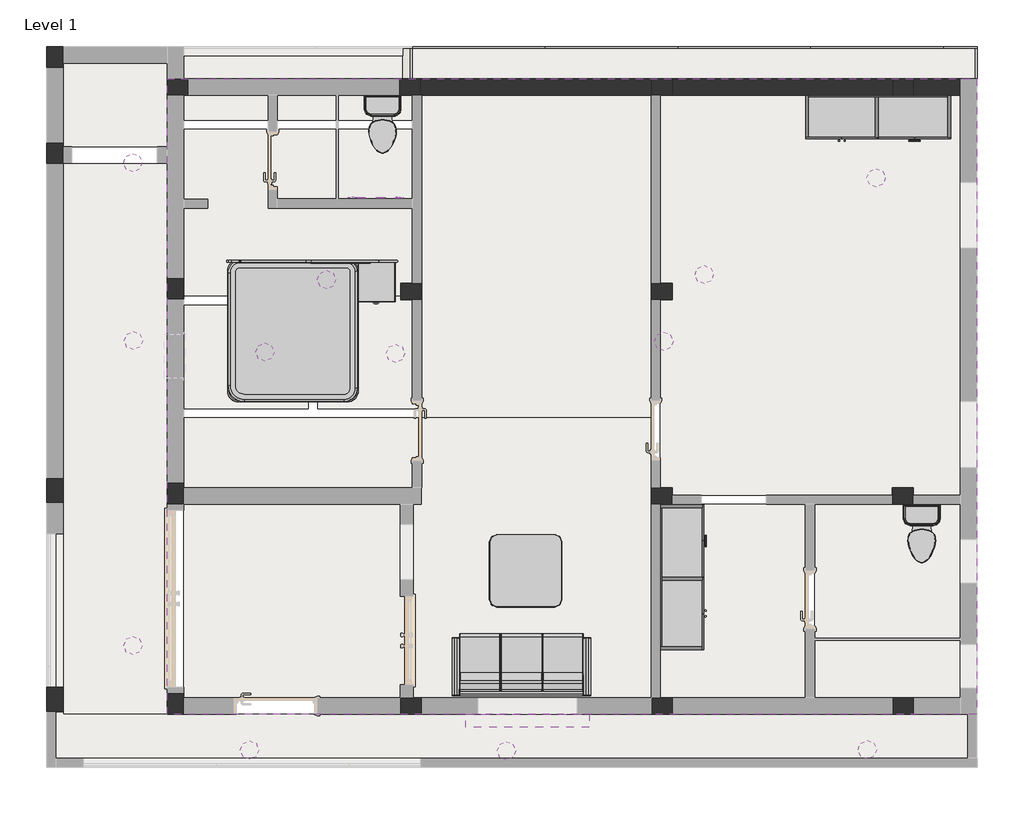
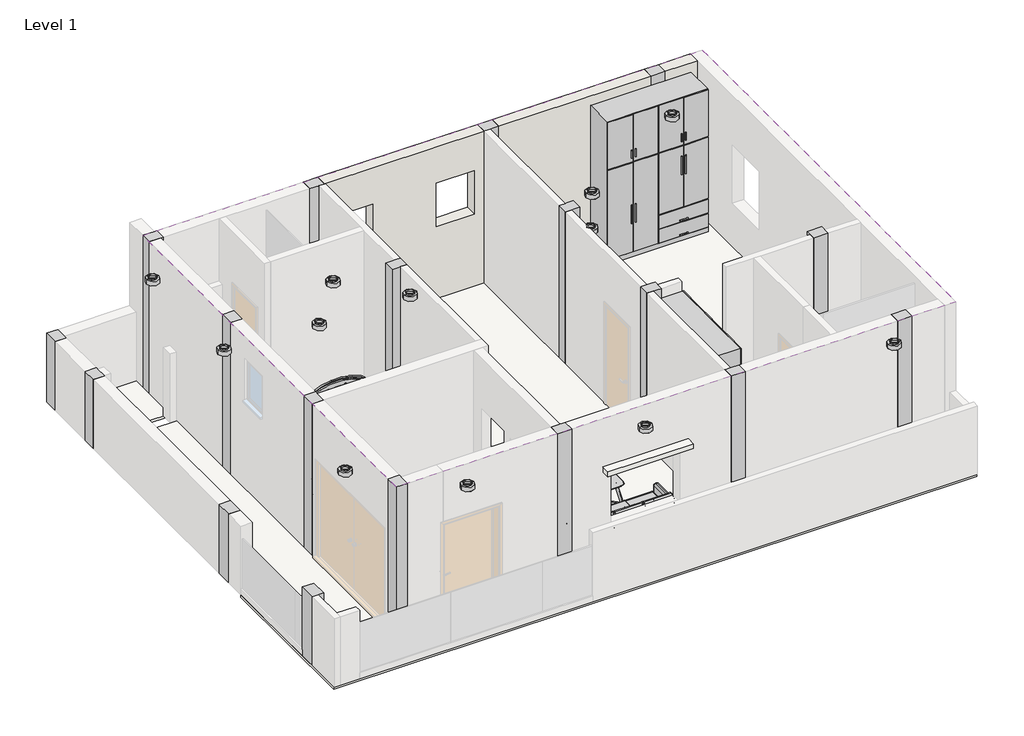
# One storey, part 2 of 2: 18 columns, 12 light fixtures, 7 plates, 6 slabs, 5 furniture elements, 4 walls, 3 flow terminals, 1 covering.
"""IFC4 building model written with IfcOpenShell, lengths in millimetres."""

from ifc_helpers import new_model, si_unit, frame, origin, place, context, project, spatial, polyline, outline, extrude, faceted_brep, transform, mapped, element, save
from components import concrete_rectangular_column_12_x_19_f479a93c, mirror_with_light_5960_af_41a2bd15, toilet_domestic_3d_toilet_domestic_3d_ba6479b0, toilet_domestic_3d_toilet_domestic_3d_30431060, furniture_2fc85b74, furniture_29a9adb8, furniture_57072a26, furniture_1wardrobe_6271_1wardrobe_6271_4dd35231, bed_design_8999_bed_design_8999_9c973422, bed_design_8999_bed_design_8999_e911dec7, coffee_table_16790_coffee_table_16790_723536ea, ceiling_light_flat_round_60w_120v_7c4c2a52, system_panel_glazed_6338a664, system_panel_glazed_bba74dcb, system_panel_glazed_77a7bb99, system_panel_glazed_06045eac

model = new_model("IFC4")

# Units and contexts
model_context = context("Model", 3, world=origin())
ifc_project = project(units=[si_unit("LENGTHUNIT", "METRE", prefix="MILLI")], contexts=[model_context])

# Site, building, storey
site = spatial("IfcSite", under=ifc_project)
building = spatial("IfcBuilding", under=site)
storey = spatial("IfcBuildingStorey", under=building, Name="Level 1", Elevation=3200.4)

# Columns
placement = place(None, origin())
element("IfcColumn", 1, ObjectType="Concrete-Rectangular-Column : 12 x 19", at=placement, inside=storey, context=model_context, shape_type="SweptSolid", body=[
    extrude(outline(polyline([(-12607.4604224, 5545.7949405), (-12607.4604224, 5253.6949405), (-12836.0604224, 5253.6949405), (-12836.0604224, 5545.7949405), (-12607.4604224, 5545.7949405)])), frame((0.0, 0.0, 3200.4), z_axis=(0.0, 0.0, 1.0), x_axis=(1.0, 0.0, 0.0)), (0.0, 0.0, 1.0), 1447.8),
])
element("IfcColumn", 2, ObjectType="Concrete-Rectangular-Column : 12 x 19", at=placement, inside=storey, context=model_context, shape_type="SweptSolid", body=[
    extrude(outline(polyline([(-12607.4604224, 4222.4988089), (-12607.4604224, 3930.3988089), (-12836.0604224, 3930.3988089), (-12836.0604224, 4222.4988089), (-12607.4604224, 4222.4988089)])), frame((0.0, 0.0, 3200.4), z_axis=(0.0, 0.0, 1.0), x_axis=(1.0, 0.0, 0.0)), (0.0, 0.0, 1.0), 1447.8),
])
element("IfcColumn", 3, ObjectType="Concrete-Rectangular-Column : 12 x 19", at=placement, inside=storey, context=model_context, shape_type="SweptSolid", body=[
    extrude(outline(polyline([(-10947.1858712, 2357.6455124), (-10947.1858712, 2065.5455124), (-11175.7858712, 2065.5455124), (-11175.7858712, 2357.6455124), (-10947.1858712, 2357.6455124)])), frame((0.0, 0.0, 3200.4), z_axis=(0.0, 0.0, 1.0), x_axis=(1.0, 0.0, 0.0)), (0.0, 0.0, 1.0), 3200.4),
])
element("IfcColumn", 4, ObjectType="Concrete-Rectangular-Column : 12 x 19", at=placement, inside=storey, context=model_context, shape_type="SweptSolid", body=[
    extrude(outline(polyline([(-10947.1858712, -467.0796054), (-10947.1858712, -759.1796054), (-11175.7858712, -759.1796054), (-11175.7858712, -467.0796054), (-10947.1858712, -467.0796054)])), frame((0.0, 0.0, 3200.4), z_axis=(0.0, 0.0, 1.0), x_axis=(1.0, 0.0, 0.0)), (0.0, 0.0, 1.0), 3200.4),
])
element("IfcColumn", 5, ObjectType="Concrete-Rectangular-Column : 12 x 19", at=placement, inside=storey, context=model_context, shape_type="Brep", body=[
    faceted_brep([(-10947.1858712, -3362.6796054, 3200.4), (-10947.1858712, -3426.1796054, 3200.4), (-10947.1858712, -3654.7796054, 3200.4), (-11175.7858712, -3654.7796054, 3200.4), (-11175.7858712, -3362.6796054, 3200.4), (-10947.1858712, -3362.6796054, 6400.8), (-10947.1858712, -3426.1796054, 6400.8), (-10947.1858712, -3654.7796054, 6400.8), (-11175.7858712, -3654.7796054, 6400.8), (-11175.7858712, -3362.6796054, 6400.8)], [[[0, 1, 2, 3, 4]], [[5, 6, 7, 2, 1, 0]], [[7, 8, 3, 2]], [[8, 9, 4, 3]], [[9, 5, 0, 4]], [[5, 9, 8, 7, 6]]]),
])
element("IfcColumn", 6, ObjectType="Concrete-Rectangular-Column : 12 x 19", at=placement, inside=storey, context=model_context, shape_type="SweptSolid", body=[
    extrude(outline(polyline([(-7668.2445565, -3654.7796054), (-7960.3445565, -3654.7796054), (-7960.3445565, -3426.1796054), (-7668.2445565, -3426.1796054), (-7668.2445565, -3654.7796054)])), frame((0.0, 0.0, 3200.4), z_axis=(0.0, 0.0, 1.0), x_axis=(1.0, 0.0, 0.0)), (0.0, 0.0, 1.0), 3200.4),
])
element("IfcColumn", 7, ObjectType="Concrete-Rectangular-Column : 12 x 19", at=placement, inside=storey, context=model_context, shape_type="SweptSolid", body=[
    extrude(outline(polyline([(-4204.83523, -3654.7796054), (-4496.93523, -3654.7796054), (-4496.93523, -3426.1796054), (-4204.83523, -3426.1796054), (-4204.83523, -3654.7796054)])), frame((0.0, 0.0, 3200.4), z_axis=(0.0, 0.0, 1.0), x_axis=(1.0, 0.0, 0.0)), (0.0, 0.0, 1.0), 3200.4),
])
element("IfcColumn", 8, ObjectType="Concrete-Rectangular-Column : 12 x 19", at=placement, inside=storey, context=model_context, shape_type="SweptSolid", body=[
    extrude(outline(polyline([(-883.78523, -3654.7796054), (-1175.88523, -3654.7796054), (-1175.88523, -3426.1796054), (-883.78523, -3426.1796054), (-883.78523, -3654.7796054)])), frame((0.0, 0.0, 3200.4), z_axis=(0.0, 0.0, 1.0), x_axis=(1.0, 0.0, 0.0)), (0.0, 0.0, 1.0), 3200.4),
])
element("IfcColumn", 9, ObjectType="Concrete-Rectangular-Column : 12 x 19", at=placement, inside=storey, context=model_context, shape_type="SweptSolid", body=[
    extrude(outline(polyline([(-890.13523, -764.1797525), (-1182.23523, -764.1797525), (-1182.23523, -535.5797525), (-890.13523, -535.5797525), (-890.13523, -764.1797525)])), frame((0.0, 0.0, 3200.4), z_axis=(0.0, 0.0, 1.0), x_axis=(1.0, 0.0, 0.0)), (0.0, 0.0, 1.0), 3200.4),
])
element("IfcColumn", 10, ObjectType="Concrete-Rectangular-Column : 12 x 19", at=placement, inside=storey, context=model_context, shape_type="SweptSolid", body=[
    extrude(outline(polyline([(-883.78523, 4873.0327475), (-1175.88523, 4873.0327475), (-1175.88523, 5101.6327475), (-883.78523, 5101.6327475), (-883.78523, 4873.0327475)])), frame((0.0, 0.0, 3200.4), z_axis=(0.0, 0.0, 1.0), x_axis=(1.0, 0.0, 0.0)), (0.0, 0.0, 1.0), 3200.4),
])
element("IfcColumn", 11, ObjectType="Concrete-Rectangular-Column : 12 x 19", at=placement, inside=storey, context=model_context, shape_type="SweptSolid", body=[
    extrude(outline(polyline([(-4207.375513, 4873.0327475), (-4499.475513, 4873.0327475), (-4499.475513, 5101.6327475), (-4207.375513, 5101.6327475), (-4207.375513, 4873.0327475)])), frame((0.0, 0.0, 3200.4), z_axis=(0.0, 0.0, 1.0), x_axis=(1.0, 0.0, 0.0)), (0.0, 0.0, 1.0), 3200.4),
])
element("IfcColumn", 12, ObjectType="Concrete-Rectangular-Column : 12 x 19", at=placement, inside=storey, context=model_context, shape_type="SweptSolid", body=[
    extrude(outline(polyline([(-7680.825513, 4873.0327475), (-7972.925513, 4873.0327475), (-7972.925513, 5101.6327475), (-7680.825513, 5101.6327475), (-7680.825513, 4873.0327475)])), frame((0.0, 0.0, 3200.4), z_axis=(0.0, 0.0, 1.0), x_axis=(1.0, 0.0, 0.0)), (0.0, 0.0, 1.0), 3200.4),
])
element("IfcColumn", 13, ObjectType="Concrete-Rectangular-Column : 12 x 19", at=placement, inside=storey, context=model_context, shape_type="SweptSolid", body=[
    extrude(outline(polyline([(-10883.6959332, 4876.8926487), (-11175.7959332, 4876.8926487), (-11175.7959332, 5105.4926487), (-10883.6959332, 5105.4926487), (-10883.6959332, 4876.8926487)])), frame((0.0, 0.0, 3200.4), z_axis=(0.0, 0.0, 1.0), x_axis=(1.0, 0.0, 0.0)), (0.0, 0.0, 1.0), 3200.4),
])
concrete_rectangular_column_12_x_19_shape = concrete_rectangular_column_12_x_19_f479a93c(model_context)
element("IfcColumn", 14, ObjectType="Concrete-Rectangular-Column : 12 x 19", at=placement, inside=storey, context=model_context, shape_type="MappedRepresentation", body=[
    mapped(concrete_rectangular_column_12_x_19_shape, transform((-7812.2134981, 2171.1077475, 0.0), x_axis=(0.0, -1.0, 0.0), y_axis=(1.0, 0.0, 0.0), z_axis=(0.0, 0.0, 1.0))),
])
element("IfcColumn", 15, ObjectType="Concrete-Rectangular-Column : 12 x 19", at=placement, inside=storey, context=model_context, shape_type="MappedRepresentation", body=[
    mapped(concrete_rectangular_column_12_x_19_shape, transform((-4360.0560272, 2171.1077475, 0.0), x_axis=(0.0, -1.0, 0.0), y_axis=(1.0, 0.0, 0.0), z_axis=(0.0, 0.0, 1.0))),
])
element("IfcColumn", 16, ObjectType="Concrete-Rectangular-Column : 12 x 19", at=placement, inside=storey, context=model_context, shape_type="MappedRepresentation", body=[
    mapped(concrete_rectangular_column_12_x_19_shape, transform((-4360.0560272, -649.8797525, 0.0), x_axis=(0.0, -1.0, 0.0), y_axis=(1.0, 0.0, 0.0), z_axis=(0.0, 0.0, 1.0))),
])
element("IfcColumn", 17, ObjectType="Concrete-Rectangular-Column : 12 x 20", at=placement, inside=storey, context=model_context, shape_type="SweptSolid", body=[
    extrude(outline(polyline([(-12607.4604224, -404.5396501), (-12607.4604224, -747.4396501), (-12836.0604224, -747.4396501), (-12836.0604224, -404.5396501), (-12607.4604224, -404.5396501)])), frame((0.0, 0.0, 3200.4), z_axis=(0.0, 0.0, 1.0), x_axis=(1.0, 0.0, 0.0)), (0.0, 0.0, 1.0), 1447.8),
])
element("IfcColumn", 18, ObjectType="Concrete-Rectangular-Column : 12 x 20", at=placement, inside=storey, context=model_context, shape_type="SweptSolid", body=[
    extrude(outline(polyline([(-12607.4604224, -3281.0896501), (-12607.4604224, -3623.9896501), (-12836.0604224, -3623.9896501), (-12836.0604224, -3281.0896501), (-12607.4604224, -3281.0896501)])), frame((0.0, 0.0, 3200.4), z_axis=(0.0, 0.0, 1.0), x_axis=(1.0, 0.0, 0.0)), (0.0, 0.0, 1.0), 1447.8),
])

# Covering
element("IfcCovering", 19, ObjectType="Plain", at=placement, inside=storey, context=model_context, shape_type="Brep", body=[
    faceted_brep([(-13.83523, 5101.6327475, 6477.0), (-11175.7858712, 5101.6327475, 6477.0), (-11175.7858712, -3654.7796054, 6477.0), (-242.43523, -3654.7796054, 6477.0), (-13.83523, -3654.7796054, 6477.0), (-13.83523, 5101.6327475, 6400.8), (-13.83523, -3654.7796054, 6400.8), (-11175.7858712, -3654.7796054, 6400.8), (-11175.7858712, 5101.6327475, 6400.8)], [[[0, 1, 2, 3, 4]], [[5, 6, 7, 8]], [[1, 0, 5, 8]], [[2, 1, 8, 7]], [[4, 3, 2, 7, 6]], [[0, 4, 6, 5]]]),
])

# Flow terminals
mirror_with_light_5960_af_shape = mirror_with_light_5960_af_41a2bd15(model_context)
element("IfcFlowTerminal", 20, ObjectType="Mirror_with_Light_5960 : AF", at=placement, inside=storey, context=model_context, shape_type="MappedRepresentation", body=[
    mapped(mirror_with_light_5960_af_shape, transform((-8322.2830614, 3383.1639975, 3505.2), x_axis=(1.0, 0.0, 0.0), y_axis=(0.0, 1.0, 0.0), z_axis=(0.0, 0.0, 1.0))),
])
toilet_domestic_3d_toilet_domestic_3d_shape = toilet_domestic_3d_toilet_domestic_3d_ba6479b0(model_context)
toilet_domestic_3d_toilet_domestic_3d_2_shape = toilet_domestic_3d_toilet_domestic_3d_30431060(model_context)
element("IfcFlowTerminal", 21, ObjectType="Toilet-Domestic-3D : Toilet-Domestic-3D", at=placement, inside=storey, context=model_context, shape_type="MappedRepresentation", body=[
    mapped(toilet_domestic_3d_toilet_domestic_3d_shape, transform((-775.83523, -1258.8757798, 3200.4), x_axis=(1.0, 0.0, 0.0), y_axis=(0.0, 1.0, 0.0), z_axis=(0.0, 0.0, 1.0))),
    mapped(toilet_domestic_3d_toilet_domestic_3d_2_shape, transform((-775.83523, -1258.8757798, 3200.4), x_axis=(1.0, 0.0, 0.0), y_axis=(0.0, 1.0, 0.0), z_axis=(0.0, 0.0, 1.0))),
])
element("IfcFlowTerminal", 22, ObjectType="Toilet-Domestic-3D : Toilet-Domestic-3D", at=placement, inside=storey, context=model_context, shape_type="MappedRepresentation", body=[
    mapped(toilet_domestic_3d_toilet_domestic_3d_shape, transform((-8205.9134981, 4382.1966213, 3200.4), x_axis=(1.0, 0.0, 0.0), y_axis=(0.0, 1.0, 0.0), z_axis=(0.0, 0.0, 1.0))),
    mapped(toilet_domestic_3d_toilet_domestic_3d_2_shape, transform((-8205.9134981, 4382.1966213, 3200.4), x_axis=(1.0, 0.0, 0.0), y_axis=(0.0, 1.0, 0.0), z_axis=(0.0, 0.0, 1.0))),
])

# Furniture
furniture_shape = furniture_2fc85b74(model_context)
furniture_2_shape = furniture_29a9adb8(model_context)
furniture_3_shape = furniture_57072a26(model_context)
element("IfcFurniture", 23, at=placement, inside=storey, context=model_context, shape_type="MappedRepresentation", body=[
    mapped(furniture_shape, transform((-6291.7541525, -2600.6796054, 3200.4), x_axis=(-1.0, 0.0, 0.0), y_axis=(0.0, -1.0, 0.0), z_axis=(0.0, 0.0, 1.0))),
    mapped(furniture_2_shape, transform((-6291.7541525, -2600.6796054, 3200.4), x_axis=(-1.0, 0.0, 0.0), y_axis=(0.0, -1.0, 0.0), z_axis=(0.0, 0.0, 1.0))),
    mapped(furniture_3_shape, transform((-6291.7541525, -2600.6796054, 3200.4), x_axis=(-1.0, 0.0, 0.0), y_axis=(0.0, -1.0, 0.0), z_axis=(0.0, 0.0, 1.0))),
])
furniture_1wardrobe_6271_1wardrobe_6271_shape = furniture_1wardrobe_6271_1wardrobe_6271_4dd35231(model_context)
element("IfcFurniture", 24, ObjectType="1Wardrobe_6271 : 1Wardrobe_6271", at=placement, inside=storey, context=model_context, shape_type="MappedRepresentation", body=[
    mapped(furniture_1wardrobe_6271_1wardrobe_6271_shape, transform((-2376.03523, 4873.0327475, 3200.4), x_axis=(1.0, 0.0, 0.0), y_axis=(0.0, 1.0, 0.0), z_axis=(0.0, 0.0, 1.0))),
])
element("IfcFurniture", 25, ObjectType="1Wardrobe_6271 : 1Wardrobe_6271", at=placement, inside=storey, context=model_context, shape_type="MappedRepresentation", body=[
    mapped(furniture_1wardrobe_6271_1wardrobe_6271_shape, transform((-4379.1060272, -2766.7129976, 3200.4), x_axis=(0.0, 1.0, 0.0), y_axis=(-1.0, 0.0, 0.0), z_axis=(0.0, 0.0, 1.0))),
])
bed_design_8999_bed_design_8999_shape = bed_design_8999_bed_design_8999_9c973422(model_context)
bed_design_8999_bed_design_8999_2_shape = bed_design_8999_bed_design_8999_e911dec7(model_context)
element("IfcFurniture", 26, ObjectType="BED_DESIGN_8999 : BED_DESIGN_8999", at=placement, inside=storey, context=model_context, shape_type="MappedRepresentation", body=[
    mapped(bed_design_8999_bed_design_8999_shape, transform((-9240.9634981, 652.6639975, 3200.4), x_axis=(1.0, 0.0, 0.0), y_axis=(0.0, 1.0, 0.0), z_axis=(0.0, 0.0, 1.0))),
    mapped(bed_design_8999_bed_design_8999_2_shape, transform((-9240.9634981, 652.6639975, 3200.4), x_axis=(1.0, 0.0, 0.0), y_axis=(0.0, 1.0, 0.0), z_axis=(0.0, 0.0, 1.0))),
])
coffee_table_16790_coffee_table_16790_shape = coffee_table_16790_coffee_table_16790_723536ea(model_context)
element("IfcFurniture", 27, ObjectType="Coffee_Table_16790 : Coffee_Table_16790", at=placement, inside=storey, context=model_context, shape_type="MappedRepresentation", body=[
    mapped(coffee_table_16790_coffee_table_16790_shape, transform((-6233.3060272, -1678.5797525, 3200.4), x_axis=(0.0, 1.0, 0.0), y_axis=(-1.0, 0.0, 0.0), z_axis=(0.0, 0.0, 1.0))),
])

# Light fixtures
ceiling_light_flat_round_60w_120v_shape = ceiling_light_flat_round_60w_120v_7c4c2a52(model_context)
element("IfcLightFixture", 28, ObjectType="Ceiling Light - Flat Round : 60W - 120V", at=placement, inside=storey, context=model_context, shape_type="MappedRepresentation", body=[
    mapped(ceiling_light_flat_round_60w_120v_shape, transform((-8976.6249266, 2333.1202007, 3962.4), x_axis=(1.0, 0.0, 0.0), y_axis=(0.0, 1.0, 0.0), z_axis=(0.0, 0.0, 1.0))),
])
element("IfcLightFixture", 29, ObjectType="Ceiling Light - Flat Round : 60W - 120V", at=placement, inside=storey, context=model_context, shape_type="MappedRepresentation", body=[
    mapped(ceiling_light_flat_round_60w_120v_shape, transform((-9826.6973698, 1336.4578052, 3962.4), x_axis=(1.0, 0.0, 0.0), y_axis=(0.0, 1.0, 0.0), z_axis=(0.0, 0.0, 1.0))),
])
element("IfcLightFixture", 30, ObjectType="Ceiling Light - Flat Round : 60W - 120V", at=placement, inside=storey, context=model_context, shape_type="MappedRepresentation", body=[
    mapped(ceiling_light_flat_round_60w_120v_shape, transform((-8027.2127557, 1317.1708554, 3962.4), x_axis=(1.0, 0.0, 0.0), y_axis=(0.0, 1.0, 0.0), z_axis=(0.0, 0.0, 1.0))),
])
element("IfcLightFixture", 31, ObjectType="Ceiling Light - Flat Round : 60W - 120V", at=placement, inside=storey, context=model_context, shape_type="MappedRepresentation", body=[
    mapped(ceiling_light_flat_round_60w_120v_shape, transform((-1403.7470603, 3737.3422943, 3962.4), x_axis=(1.0, 0.0, 0.0), y_axis=(0.0, 1.0, 0.0), z_axis=(0.0, 0.0, 1.0))),
])
element("IfcLightFixture", 32, ObjectType="Ceiling Light - Flat Round : 60W - 120V", at=placement, inside=storey, context=model_context, shape_type="MappedRepresentation", body=[
    mapped(ceiling_light_flat_round_60w_120v_shape, transform((-4329.6170331, 1484.2886755, 3962.4), x_axis=(1.0, 0.0, 0.0), y_axis=(0.0, 1.0, 0.0), z_axis=(0.0, 0.0, 1.0))),
])
element("IfcLightFixture", 33, ObjectType="Ceiling Light - Flat Round : 60W - 120V", at=placement, inside=storey, context=model_context, shape_type="MappedRepresentation", body=[
    mapped(ceiling_light_flat_round_60w_120v_shape, transform((-3772.5595971, 2403.8335381, 3962.4), x_axis=(1.0, 0.0, 0.0), y_axis=(0.0, 1.0, 0.0), z_axis=(0.0, 0.0, 1.0))),
])
element("IfcLightFixture", 34, ObjectType="Ceiling Light - Flat Round : 60W - 277V", at=placement, inside=storey, context=model_context, shape_type="MappedRepresentation", body=[
    mapped(ceiling_light_flat_round_60w_120v_shape, transform((-11647.8170744, 3944.8565115, 3962.4), x_axis=(1.0, 0.0, 0.0), y_axis=(0.0, 1.0, 0.0), z_axis=(0.0, 0.0, 1.0))),
])
element("IfcLightFixture", 35, ObjectType="Ceiling Light - Flat Round : 60W - 277V", at=placement, inside=storey, context=model_context, shape_type="MappedRepresentation", body=[
    mapped(ceiling_light_flat_round_60w_120v_shape, transform((-11638.1699852, 1493.9262651, 3962.4), x_axis=(1.0, 0.0, 0.0), y_axis=(0.0, 1.0, 0.0), z_axis=(0.0, 0.0, 1.0))),
])
element("IfcLightFixture", 36, ObjectType="Ceiling Light - Flat Round : 60W - 277V", at=placement, inside=storey, context=model_context, shape_type="MappedRepresentation", body=[
    mapped(ceiling_light_flat_round_60w_120v_shape, transform((-11644.9561662, -2707.9806169, 3962.4), x_axis=(1.0, 0.0, 0.0), y_axis=(0.0, 1.0, 0.0), z_axis=(0.0, 0.0, 1.0))),
])
element("IfcLightFixture", 37, ObjectType="Ceiling Light - Flat Round : 60W - 277V", at=placement, inside=storey, context=model_context, shape_type="MappedRepresentation", body=[
    mapped(ceiling_light_flat_round_60w_120v_shape, transform((-10037.5878836, -4148.1202674, 3962.4), x_axis=(1.0, 0.0, 0.0), y_axis=(0.0, 1.0, 0.0), z_axis=(0.0, 0.0, 1.0))),
])
element("IfcLightFixture", 38, ObjectType="Ceiling Light - Flat Round : 60W - 277V", at=placement, inside=storey, context=model_context, shape_type="MappedRepresentation", body=[
    mapped(ceiling_light_flat_round_60w_120v_shape, transform((-6498.1676871, -4159.8217019, 3962.4), x_axis=(1.0, 0.0, 0.0), y_axis=(0.0, 1.0, 0.0), z_axis=(0.0, 0.0, 1.0))),
])
element("IfcLightFixture", 39, ObjectType="Ceiling Light - Flat Round : 60W - 277V", at=placement, inside=storey, context=model_context, shape_type="MappedRepresentation", body=[
    mapped(ceiling_light_flat_round_60w_120v_shape, transform((-1525.3967065, -4143.4135843, 3962.4), x_axis=(1.0, 0.0, 0.0), y_axis=(0.0, 1.0, 0.0), z_axis=(0.0, 0.0, 1.0))),
])

# Plates
system_panel_glazed_shape = system_panel_glazed_6338a664(model_context)
element("IfcPlate", 40, ObjectType="System Panel : Glazed", at=placement, inside=storey, context=model_context, shape_type="MappedRepresentation", body=[
    mapped(system_panel_glazed_shape, transform((-6883.885871, 5497.0125322, 3200.4), x_axis=(1.0, 0.0, 0.0), y_axis=(0.0, 1.0, 0.0), z_axis=(0.0, 0.0, 1.0))),
])
element("IfcPlate", 41, ObjectType="System Panel : Glazed", at=placement, inside=storey, context=model_context, shape_type="MappedRepresentation", body=[
    mapped(system_panel_glazed_shape, transform((-5053.8858709, 5497.0125322, 3200.4), x_axis=(1.0, 0.0, 0.0), y_axis=(0.0, 1.0, 0.0), z_axis=(0.0, 0.0, 1.0))),
])
element("IfcPlate", 42, ObjectType="System Panel : Glazed", at=placement, inside=storey, context=model_context, shape_type="MappedRepresentation", body=[
    mapped(system_panel_glazed_shape, transform((-3223.8858709, 5497.0125322, 3200.4), x_axis=(1.0, 0.0, 0.0), y_axis=(0.0, 1.0, 0.0), z_axis=(0.0, 0.0, 1.0))),
])
element("IfcPlate", 43, ObjectType="System Panel : Glazed", at=placement, inside=storey, context=model_context, shape_type="MappedRepresentation", body=[
    mapped(system_panel_glazed_shape, transform((-1393.8858709, 5497.0125322, 3200.4), x_axis=(1.0, 0.0, 0.0), y_axis=(0.0, 1.0, 0.0), z_axis=(0.0, 0.0, 1.0))),
])
system_panel_glazed_2_shape = system_panel_glazed_bba74dcb(model_context)
element("IfcPlate", 44, ObjectType="System Panel : Glazed", at=placement, inside=storey, context=model_context, shape_type="MappedRepresentation", body=[
    mapped(system_panel_glazed_2_shape, transform((-7848.3858712, 5311.357594, 3200.4), x_axis=(0.0, -1.0, 0.0), y_axis=(1.0, 0.0, 0.0), z_axis=(0.0, 0.0, 1.0))),
])
system_panel_glazed_3_shape = system_panel_glazed_77a7bb99(model_context)
element("IfcPlate", 45, ObjectType="System Panel : Glazed", at=placement, inside=storey, context=model_context, shape_type="MappedRepresentation", body=[
    mapped(system_panel_glazed_3_shape, transform((-244.8620085, 5497.0125322, 3200.4), x_axis=(1.0, 0.0, 0.0), y_axis=(0.0, 1.0, 0.0), z_axis=(0.0, 0.0, 1.0))),
])
system_panel_glazed_4_shape = system_panel_glazed_06045eac(model_context)
element("IfcPlate", 46, ObjectType="System Panel : Glazed", at=placement, inside=storey, context=model_context, shape_type="MappedRepresentation", body=[
    mapped(system_panel_glazed_4_shape, transform((-60.3381462, 5311.5726399, 3200.4), x_axis=(0.0, -1.0, 0.0), y_axis=(1.0, 0.0, 0.0), z_axis=(0.0, 0.0, 1.0))),
])

# Slabs
element("IfcSlab", 47, ObjectType="2\"", at=placement, inside=storey, context=model_context, shape_type="SweptSolid", body=[
    extrude(outline(polyline([(-11175.7858712, 5317.1949405), (-11175.7858712, 4168.5238089), (-12610.0019081, 4168.5238089), (-12610.0019081, 5317.1949405), (-11175.7858712, 5317.1949405)])), frame((0.0, 0.0, 3149.6), z_axis=(0.0, 0.0, 1.0), x_axis=(1.0, 0.0, 0.0)), (0.0, 0.0, 1.0), 50.8),
    extrude(outline(polyline([(-11175.7858712, 3930.3988089), (-11175.7858712, -3654.7796054), (-12607.4604224, -3654.7796054), (-12607.4604224, 3930.3988089), (-11175.7858712, 3930.3988089)])), frame((0.0, 0.0, 3149.6), z_axis=(0.0, 0.0, 1.0), x_axis=(1.0, 0.0, 0.0)), (0.0, 0.0, 1.0), 50.8),
    extrude(outline(polyline([(-7793.1634981, 4403.8176487), (-7793.1634981, 2285.4077475), (-7958.2634981, 2285.4077475), (-7958.2634981, 2110.7280605), (-10947.1858712, 2110.7280605), (-10947.1858712, 4403.8176487), (-7793.1634981, 4403.8176487)])), frame((0.0, 0.0, 3149.6), z_axis=(0.0, 0.0, 1.0), x_axis=(1.0, 0.0, 0.0)), (0.0, 0.0, 1.0), 50.8),
    extrude(outline(polyline([(-9226.3358712, 1983.7280605), (-9226.3358712, 555.2703946), (-10947.1858712, 555.2703946), (-10947.1858712, 1983.7280605), (-9226.3358712, 1983.7280605)])), frame((0.0, 0.0, 3149.6), z_axis=(0.0, 0.0, 1.0), x_axis=(1.0, 0.0, 0.0)), (0.0, 0.0, 1.0), 50.8),
    extrude(outline(polyline([(-4506.1060272, 428.2703946), (-4506.1060272, -3426.1796054), (-10947.1858712, -3426.1796054), (-10947.1858712, 428.2703946), (-4506.1060272, 428.2703946)])), frame((0.0, 0.0, 3149.6), z_axis=(0.0, 0.0, 1.0), x_axis=(1.0, 0.0, 0.0)), (0.0, 0.0, 1.0), 50.8),
    extrude(outline(polyline([(-242.43523, 4873.0327475), (-242.43523, -637.1797525), (-890.13523, -637.1797525), (-890.13523, -535.5797525), (-1182.23523, -535.5797525), (-1182.23523, -637.1797525), (-3948.1683882, -637.1797525), (-4214.0060272, -637.1797525), (-4214.0060272, -535.5797525), (-4379.1060272, -535.5797525), (-4379.1060272, 2056.8077475), (-4214.0060272, 2056.8077475), (-4214.0060272, 2285.4077475), (-4379.1060272, 2285.4077475), (-4379.1060272, 4873.0327475), (-242.43523, 4873.0327475)])), frame((0.0, 0.0, 3149.6), z_axis=(0.0, 0.0, 1.0), x_axis=(1.0, 0.0, 0.0)), (0.0, 0.0, 1.0), 50.8),
    extrude(outline(polyline([(-2378.5983223, -764.1797525), (-2378.5983223, -3426.1796054), (-4379.1060272, -3426.1796054), (-4379.1060272, -764.1797525), (-2378.5983223, -764.1797525)])), frame((0.0, 0.0, 3149.6), z_axis=(0.0, 0.0, 1.0), x_axis=(1.0, 0.0, 0.0)), (0.0, 0.0, 1.0), 50.8),
    extrude(outline(polyline([(-242.43523, -764.1797525), (-242.43523, -3426.1796054), (-2251.5983223, -3426.1796054), (-2251.5983223, -764.1797525), (-242.43523, -764.1797525)])), frame((0.0, 0.0, 3149.6), z_axis=(0.0, 0.0, 1.0), x_axis=(1.0, 0.0, 0.0)), (0.0, 0.0, 1.0), 50.8),
])
element("IfcSlab", 48, ObjectType="2\"", at=placement, inside=storey, context=model_context, shape_type="SweptSolid", body=[
    extrude(outline(polyline([(-7958.2634981, 2110.7280605), (-7958.2634981, 2056.8077475), (-7666.1634981, 2056.8077475), (-7666.1634981, 4869.8577475), (-4506.1060272, 4869.8577475), (-4506.1060272, 2086.6253561), (-4506.1060272, 428.2703946), (-7670.5858712, 428.2703946), (-7670.5858712, 555.2703946), (-9099.7845381, 555.2703946), (-9099.7845381, 2110.7280605), (-7958.2634981, 2110.7280605)])), frame((0.0, 0.0, 3149.6), z_axis=(0.0, 0.0, 1.0), x_axis=(1.0, 0.0, 0.0)), (0.0, 0.0, 1.0), 50.8),
])
element("IfcSlab", 49, ObjectType="2\"", at=placement, inside=storey, context=model_context, shape_type="SweptSolid", body=[
    extrude(outline(polyline([(-7798.8858712, 5496.5824405), (-7798.8858712, 5101.6327475), (-7972.925513, 5101.6327475), (-7972.925513, 4873.0327475), (-7793.1634981, 4873.0327475), (-7793.1634981, 4530.8176487), (-10947.1858712, 4530.8176487), (-10947.1858712, 4876.8926487), (-10883.6959332, 4876.8926487), (-10883.6959332, 5105.4926487), (-10947.1858712, 5105.4926487), (-10947.1858712, 5496.5824405), (-7798.8858712, 5496.5824405)])), frame((0.0, 0.0, 3149.6), z_axis=(0.0, 0.0, 1.0), x_axis=(1.0, 0.0, 0.0)), (0.0, 0.0, 1.0), 50.8),
])
element("IfcSlab", 50, ObjectType="2\"", at=placement, inside=storey, context=model_context, shape_type="SweptSolid", body=[
    extrude(outline(polyline([(-35.8381462, 5521.0824405), (-35.8381462, 5101.6327475), (-7798.8858712, 5101.6327475), (-7798.8858712, 5521.0824405), (-35.8381462, 5521.0824405)])), frame((0.0, 0.0, 3149.6), z_axis=(0.0, 0.0, 1.0), x_axis=(1.0, 0.0, 0.0)), (0.0, 0.0, 1.0), 50.8),
])
element("IfcSlab", 51, ObjectType="2\"", at=placement, inside=storey, context=model_context, shape_type="SweptSolid", body=[
    extrude(outline(polyline([(-12836.0604224, -4367.455056), (-12836.0604224, -1167.055056), (-12607.4604224, -1167.055056), (-12607.4604224, -3654.7796054), (-12110.227509, -3654.7796054), (-13.83523, -3654.7796054), (-13.83523, -4367.455056), (-12836.0604224, -4367.455056)])), frame((0.0, 0.0, 3149.6), z_axis=(0.0, 0.0, 1.0), x_axis=(1.0, 0.0, 0.0)), (0.0, 0.0, 1.0), 50.8),
])
element("IfcSlab", 52, ObjectType="2\" 2", at=placement, inside=storey, context=model_context, shape_type="SweptSolid", body=[
    extrude(outline(polyline([(189.36477, 3834.9017586), (189.36477, 2615.7017586), (-13.83523, 2615.7017586), (-13.83523, 3834.9017586), (189.36477, 3834.9017586)])), frame((0.0, 0.0, 5283.2), z_axis=(0.0, 0.0, 1.0), x_axis=(1.0, 0.0, 0.0)), (0.0, 0.0, 1.0), 101.6),
    extrude(outline(polyline([(189.36477, 812.3017586), (189.36477, -406.8982414), (-13.83523, -406.8982414), (-13.83523, 812.3017586), (189.36477, 812.3017586)])), frame((0.0, 0.0, 5283.2), z_axis=(0.0, 0.0, 1.0), x_axis=(1.0, 0.0, 0.0)), (0.0, 0.0, 1.0), 101.6),
    extrude(outline(polyline([(138.56477, -1561.9088941), (138.56477, -2400.1088941), (-13.83523, -2400.1088941), (-13.83523, -1561.9088941), (138.56477, -1561.9088941)])), frame((0.0, 0.0, 5283.2), z_axis=(0.0, 0.0, 1.0), x_axis=(1.0, 0.0, 0.0)), (0.0, 0.0, 1.0), 101.6),
    extrude(outline(polyline([(-5355.4207599, -3654.7796054), (-5355.4207599, -3832.5796054), (-7057.2207599, -3832.5796054), (-7057.2207599, -3654.7796054), (-5355.4207599, -3654.7796054)])), frame((0.0, 0.0, 5283.2), z_axis=(0.0, 0.0, 1.0), x_axis=(1.0, 0.0, 0.0)), (0.0, 0.0, 1.0), 101.6),
])

# Walls
element("IfcWall", 53, ObjectType="5\"", at=placement, inside=storey, context=model_context, shape_type="Brep", body=[
    faceted_brep([(-7926.5134981, 5546.4824405, 3200.4), (-7926.5134981, 5419.4824405, 3200.4), (-7926.5134981, 5101.6327475, 3200.4), (-7926.5134981, 5101.6327475, 3276.6), (-7926.5134981, 5419.4824405, 3276.6), (-7926.5134981, 5546.4824405, 3276.6), (-7799.5134981, 5546.4824405, 3200.4), (-7799.5134981, 5546.4824405, 3276.6), (-7799.5134981, 5101.6327475, 3276.6), (-7799.5134981, 5101.6327475, 3200.4)], [[[0, 1, 2, 3, 4, 5]], [[6, 7, 8, 9]], [[2, 1, 0, 6, 9]], [[3, 2, 9, 8]], [[5, 4, 3, 8, 7]], [[0, 5, 7, 6]]]),
])
element("IfcWall", 54, ObjectType="9\"", at=placement, inside=storey, context=model_context, shape_type="SweptSolid", body=[
    extrude(outline(polyline([(-883.78523, 5101.6327475), (-242.43523, 5101.6327475), (-242.43523, 4873.0327475), (-883.78523, 4873.0327475), (-883.78523, 5101.6327475)])), frame((0.0, 0.0, 3200.4), z_axis=(0.0, 0.0, 1.0), x_axis=(1.0, 0.0, 0.0)), (0.0, 0.0, 1.0), 3200.4),
])
element("IfcWall", 55, ObjectType="9\"", at=placement, inside=storey, context=model_context, shape_type="SweptSolid", body=[
    extrude(outline(polyline([(-4207.375513, 5101.6327475), (-1175.88523, 5101.6327475), (-1175.88523, 4873.0327475), (-4207.375513, 4873.0327475), (-4207.375513, 5101.6327475)])), frame((0.0, 0.0, 3200.4), z_axis=(0.0, 0.0, 1.0), x_axis=(1.0, 0.0, 0.0)), (0.0, 0.0, 1.0), 3200.4),
])
element("IfcWall", 56, ObjectType="9\"", at=placement, inside=storey, context=model_context, shape_type="Brep", body=[
    faceted_brep([(-4499.475513, 5101.6327475, 3200.4), (-7680.825513, 5101.6327475, 3200.4), (-7680.825513, 5101.6327475, 6400.8), (-4499.475513, 5101.6327475, 6400.8), (-7477.625513, 5101.6327475, 5638.8), (-7477.625513, 5101.6327475, 4724.4), (-6715.625513, 5101.6327475, 4724.4), (-6715.625513, 5101.6327475, 5638.8), (-5458.325513, 5101.6327475, 5638.8), (-5458.325513, 5101.6327475, 4724.4), (-4696.325513, 5101.6327475, 4724.4), (-4696.325513, 5101.6327475, 5638.8), (-4499.475513, 4873.0327475, 3200.4), (-4499.475513, 4873.0327475, 6400.8), (-7666.1634981, 4873.0327475, 6400.8), (-7680.825513, 4873.0327475, 6400.8), (-7680.825513, 4873.0327475, 3200.4), (-7666.1634981, 4873.0327475, 3200.4), (-7477.625513, 4873.0327475, 5638.8), (-6715.625513, 4873.0327475, 5638.8), (-6715.625513, 4873.0327475, 4724.4), (-7477.625513, 4873.0327475, 4724.4), (-5458.325513, 4873.0327475, 5638.8), (-4696.325513, 4873.0327475, 5638.8), (-4696.325513, 4873.0327475, 4724.4), (-5458.325513, 4873.0327475, 4724.4)], [[[0, 1, 2, 3], [4, 5, 6, 7], [8, 9, 10, 11]], [[12, 13, 14, 15, 16, 17], [18, 19, 20, 21], [22, 23, 24, 25]], [[1, 0, 12, 17, 16]], [[2, 1, 16, 15]], [[3, 2, 15, 14, 13]], [[0, 3, 13, 12]], [[5, 4, 18, 21]], [[6, 5, 21, 20]], [[7, 6, 20, 19]], [[4, 7, 19, 18]], [[9, 8, 22, 25]], [[10, 9, 25, 24]], [[11, 10, 24, 23]], [[8, 11, 23, 22]]]),
])

save(model, "model.ifc")

# Revit data of these elements
# Type "Concrete-Rectangular-Column : 12 x 19"
#   Assembly Code = "B10"
#   b = 0' - 9"
#   h = 0' - 11 1/2"
#   Structural Material [instance default] = Concrete, Cast-in-Place gray
# Type "Concrete-Rectangular-Column : 12 x 20"
#   Assembly Code = "B10"
#   b = 0' - 9"
#   h = 1' - 1 1/2"
#   Structural Material [instance default] = Concrete, Cast-in-Place gray
# Type "Plain"
#   Keynote = "K40"
#   built-in parameter 1002203 = 1 (stored number, unit not read)
#   built-in parameter 1002202 = 1 (stored number, unit not read)
#   Layers, outside or top first: 0' - 3" "Metal Stud Layer" (function 1)
# Type "Mirror_with_Light_5960 : AF"
#   Width [instance default] = 2' - 6"
#   Sill Hight [instance default] = 4' - 0"
#   Mirror Height = 3' - 0"
#   Depth [instance default] = 0' - 1"
#   Default Elevation = 0
#   Assembly Code = ""
# Type "Toilet-Domestic-3D : Toilet-Domestic-3D"
#   Assembly Code = "D2010110"
#   Toilet - Bowl/Basin Material = Porcelain, Linen
#   Toilet - Seat Material = Laminate, Linen, Matte
#   Default Elevation = 0
# Type
#   Width [instance] = 6' - 3.19685"
#   Default Elevation = 0
# Type "1Wardrobe_6271 : 1Wardrobe_6271"
#   Default Elevation = 0
# Type "BED_DESIGN_8999 : BED_DESIGN_8999"
#   Default Elevation = 0
# Type "Coffee_Table_16790 : Coffee_Table_16790"
#   Coffee Table - Stand = Coffee Table - Stand
#   Coffee Table - Glass = Coffee Table - Glass
#   Default Elevation = 0
# Type "Ceiling Light - Flat Round : 60W - 120V"
#   Lamp = "A-19"
#   Assembly Code = "D5020220"
#   Wattage = 60 W
#   built-in parameter 1150110 = 1 (stored number, unit not read)
#   built-in parameter 1114217 = 1 (stored number, unit not read)
#   built-in parameter 1150109 = 1 (stored number, unit not read)
#   built-in parameter 1150113 = 1 (stored number, unit not read)
#   built-in parameter 1150115 = 1 (stored number, unit not read)
#   built-in parameter 1150105 = 272.155 (stored number, unit not read)
#   Light Source Symbol Size = 2' - 0"
#   built-in parameter 1150112 = 1 (stored number, unit not read)
#   built-in parameter 1150114 = 1 (stored number, unit not read)
#   built-in parameter 1150107 = 2800 (stored number, unit not read)
#   built-in parameter 1150106 = 2.72155 (stored number, unit not read)
#   Emit from Circle Diameter = 0' - 10"
#   built-in parameter 1150104 = 1.32387 (stored number, unit not read)
#   Ballast Voltage = 120 V
#   built-in parameter 1114218 = 1 (stored number, unit not read)
#   built-in parameter 1150133 = 10 (stored number, unit not read)
#   Lumens = 855 lm
#   Apparent Load = 60 VA
#   built-in parameter 1150134 = 4
#   built-in parameter 1150137 = 1
#   Color Filter = 16777215
#   built-in parameter 1140040 [instance default] = 1
#   Ballast Number of Poles = 1
#   Light Box Material = Steel, Paint Finish, Dark Gray, Matte
#   Diffuser Material = Glass, White, High Luminance
#   Wattage Comments = ""
#   Emit Shape Visible in Rendering = no
#   Dimming Lamp Color Temperature Shift = (empty or 0)
#   Default Elevation = 0
# Type "Ceiling Light - Flat Round : 60W - 277V"
#   Lamp = "A-19"
#   Assembly Code = "D5020220"
#   Wattage = 60 W
#   built-in parameter 1150110 = 1 (stored number, unit not read)
#   built-in parameter 1114217 = 1 (stored number, unit not read)
#   built-in parameter 1150109 = 1 (stored number, unit not read)
#   built-in parameter 1150113 = 1 (stored number, unit not read)
#   built-in parameter 1150115 = 1 (stored number, unit not read)
#   built-in parameter 1150105 = 272.155 (stored number, unit not read)
#   Light Source Symbol Size = 2' - 0"
#   built-in parameter 1150112 = 1 (stored number, unit not read)
#   built-in parameter 1150114 = 1 (stored number, unit not read)
#   built-in parameter 1150107 = 2800 (stored number, unit not read)
#   built-in parameter 1150106 = 2.72155 (stored number, unit not read)
#   Emit from Circle Diameter = 0' - 10"
#   built-in parameter 1150104 = 1.32387 (stored number, unit not read)
#   Ballast Voltage = 277 V
#   built-in parameter 1114218 = 1 (stored number, unit not read)
#   built-in parameter 1150133 = 10 (stored number, unit not read)
#   Lumens = 855 lm
#   Apparent Load = 60 VA
#   built-in parameter 1150134 = 4
#   built-in parameter 1150137 = 1
#   Color Filter = 16777215
#   built-in parameter 1140040 [instance default] = 1
#   Ballast Number of Poles = 1
#   Light Box Material = Steel, Paint Finish, Dark Gray, Matte
#   Diffuser Material = Glass, White, High Luminance
#   Wattage Comments = ""
#   Emit Shape Visible in Rendering = no
#   Dimming Lamp Color Temperature Shift = (empty or 0)
#   Default Elevation = 0
# Type "System Panel : Glazed"
#   Keynote = "H11"
#   Construction Type Id = "GSP4R"
#   Analytic Construction = "1/8 in Pilkington single glazing"
#   Visual Light Transmittance = 0.9
#   Solar Heat Gain Coefficient = 0.86
#   Heat Transfer Coefficient (U) = 6.7069 W/(m²·K)
#   Define Thermal Properties by = 1
# Type "2\""
#   Function = 0
#   Layers, outside or top first: 0' - 2" "Concrete, Cast-in-Place - C15" (function 1)
# Type "2\" 2"
#   Function = 0
#   Layers, outside or top first: 0' - 4" "Concrete, Cast-in-Place - C15" (function 1)
# Type "5\""
#   Keynote = "F10"
#   Layers, outside or top first: 0' - 5" "Concrete" (function 1)
# Type "9\""
#   Keynote = "F10"
#   Layers, outside or top first: 0' - 9" "Concrete" (function 1)
# Elements 1, 2, 3, 4, 6, 7, 8, 10, 11, 13 (IfcColumn, "Concrete-Rectangular-Column : 12 x 19")
#   Structural Material = Concrete Masonry Units
#   Phase Created = New Construction
#   Materials on its faces: "Concrete Masonry Units", "Gypsum Wall Board"
# Element 5 (IfcColumn, "Concrete-Rectangular-Column : 12 x 19")
#   Structural Material = Concrete Masonry Units
#   Phase Created = New Construction
#   Materials on its faces: "Concrete Masonry Units", "new"
# Elements 9, 12, 14, 15, 16 (IfcColumn, "Concrete-Rectangular-Column : 12 x 19")
#   Structural Material = Concrete Masonry Units
#   Phase Created = New Construction
#   Materials on its faces: "Concrete Masonry Units"
# Element 17 (IfcColumn, "Concrete-Rectangular-Column : 12 x 20")
#   Structural Material = Concrete Masonry Units
#   Phase Created = New Construction
#   Materials on its faces: "Concrete Masonry Units", "Gypsum Wall Board"
# Element 18 (IfcColumn, "Concrete-Rectangular-Column : 12 x 20")
#   Structural Material = Concrete Masonry Units
#   Phase Created = New Construction
#   Materials on its faces: "Concrete Masonry Units", "Liquid - White Wine"
# Element 19 (IfcCovering, "Plain")
#   Height Offset From Level = 10' - 6"
#   Phase Created = New Construction
#   Materials on its faces: "Metal Stud Layer", "Gypsum Wall Board"
# Element 20 (IfcFlowTerminal, "Mirror_with_Light_5960 : AF")
#   Mark = "6"
#   Width = 2' - 6"
#   Sill Hight = 4' - 0"
#   Depth = 0' - 1"
#   Phase Created = New Construction
#   Materials on its faces: "Metal", "Glass 2", "Glass"
# Element 21 (IfcFlowTerminal, "Toilet-Domestic-3D : Toilet-Domestic-3D")
#   Mark = "2"
#   Phase Created = New Construction
#   Materials on its faces: "Porcelain, Linen", "Laminate, Linen, Matte"
# Element 22 (IfcFlowTerminal, "Toilet-Domestic-3D : Toilet-Domestic-3D")
#   Mark = "4"
#   Phase Created = New Construction
#   Materials on its faces: "Porcelain, Linen", "Laminate, Linen, Matte"
# Element 23 (IfcFurniture)
#   Width = 6' - 6.37253"
#   Phase Created = New Construction
# Elements 24, 25 (IfcFurniture, "1Wardrobe_6271 : 1Wardrobe_6271")
#   Phase Created = New Construction
#   Materials on its faces: "Phase - Demo", "Default Wall", "Phase - Exist", "Default"
# Element 26 (IfcFurniture, "BED_DESIGN_8999 : BED_DESIGN_8999")
#   Phase Created = New Construction
#   Materials on its faces: "wood 2", "ss", "new wood", "fabric 2", "wood light", "fabric"
# Element 27 (IfcFurniture, "Coffee_Table_16790 : Coffee_Table_16790")
#   Phase Created = New Construction
#   Materials on its faces: "Coffee Table - Stand", "Coffee Table - Glass"
# Element 28 (IfcLightFixture, "Ceiling Light - Flat Round : 60W - 120V")
#   Mark = "1"
#   built-in parameter 1140040 = 1
#   Phase Created = New Construction
#   Materials on its faces: "Glass, White, High Luminance", "Steel, Paint Finish, Dark Gray, Matte"
# Element 29 (IfcLightFixture, "Ceiling Light - Flat Round : 60W - 120V")
#   Mark = "2"
#   built-in parameter 1140040 = 1
#   Phase Created = New Construction
#   Materials on its faces: "Glass, White, High Luminance", "Steel, Paint Finish, Dark Gray, Matte"
# Element 30 (IfcLightFixture, "Ceiling Light - Flat Round : 60W - 120V")
#   Mark = "3"
#   built-in parameter 1140040 = 1
#   Phase Created = New Construction
#   Materials on its faces: "Glass, White, High Luminance", "Steel, Paint Finish, Dark Gray, Matte"
# Element 31 (IfcLightFixture, "Ceiling Light - Flat Round : 60W - 120V")
#   Mark = "4"
#   built-in parameter 1140040 = 1
#   Phase Created = New Construction
#   Materials on its faces: "Glass, White, High Luminance", "Steel, Paint Finish, Dark Gray, Matte"
# Element 32 (IfcLightFixture, "Ceiling Light - Flat Round : 60W - 120V")
#   Mark = "5"
#   built-in parameter 1140040 = 1
#   Phase Created = New Construction
#   Materials on its faces: "Glass, White, High Luminance", "Steel, Paint Finish, Dark Gray, Matte"
# Element 33 (IfcLightFixture, "Ceiling Light - Flat Round : 60W - 120V")
#   Mark = "6"
#   built-in parameter 1140040 = 1
#   Phase Created = New Construction
#   Materials on its faces: "Glass, White, High Luminance", "Steel, Paint Finish, Dark Gray, Matte"
# Element 34 (IfcLightFixture, "Ceiling Light - Flat Round : 60W - 277V")
#   Mark = "7"
#   built-in parameter 1140040 = 1
#   Phase Created = New Construction
#   Materials on its faces: "Glass, White, High Luminance", "Steel, Paint Finish, Dark Gray, Matte"
# Element 35 (IfcLightFixture, "Ceiling Light - Flat Round : 60W - 277V")
#   Mark = "8"
#   built-in parameter 1140040 = 1
#   Phase Created = New Construction
#   Materials on its faces: "Glass, White, High Luminance", "Steel, Paint Finish, Dark Gray, Matte"
# Element 36 (IfcLightFixture, "Ceiling Light - Flat Round : 60W - 277V")
#   Mark = "9"
#   built-in parameter 1140040 = 1
#   Phase Created = New Construction
#   Materials on its faces: "Glass, White, High Luminance", "Steel, Paint Finish, Dark Gray, Matte"
# Element 37 (IfcLightFixture, "Ceiling Light - Flat Round : 60W - 277V")
#   Mark = "10"
#   built-in parameter 1140040 = 1
#   Phase Created = New Construction
#   Materials on its faces: "Glass, White, High Luminance", "Steel, Paint Finish, Dark Gray, Matte"
# Element 38 (IfcLightFixture, "Ceiling Light - Flat Round : 60W - 277V")
#   Mark = "11"
#   built-in parameter 1140040 = 1
#   Phase Created = New Construction
#   Materials on its faces: "Glass, White, High Luminance", "Steel, Paint Finish, Dark Gray, Matte"
# Element 39 (IfcLightFixture, "Ceiling Light - Flat Round : 60W - 277V")
#   Mark = "12"
#   built-in parameter 1140040 = 1
#   Phase Created = New Construction
#   Materials on its faces: "Glass, White, High Luminance", "Steel, Paint Finish, Dark Gray, Matte"
# Elements 40, 41, 42, 43, 44, 45, 46 (IfcPlate, "System Panel : Glazed")
#   Phase Created = New Construction
#   Materials on its faces: "Glass"
# Elements 47, 48, 49, 50 (IfcSlab, "2\"")
#   Height Offset From Level = 0' - 0"
#   Phase Created = New Construction
#   Materials on its faces: "Concrete, Cast-in-Place - C15"
# Element 51 (IfcSlab, "2\"")
#   built-in parameter 1001955 = -1.5708 (stored number, unit not read)
#   Height Offset From Level = 0' - 0"
#   Phase Created = New Construction
#   Materials on its faces: "Concrete, Cast-in-Place - C15", "Liquid - White Wine"
# Element 52 (IfcSlab, "2\" 2")
#   Height Offset From Level = 7' - 2"
#   Phase Created = New Construction
#   Materials on its faces: "Concrete, Cast-in-Place - C15"
# Element 53 (IfcWall, "5\"")
#   Top Offset = 0' - 0"
#   Base Offset = 0' - 0"
#   Unconnected Height = 0' - 3"
#   wall height = 0' - 3"
#   Phase Created = New Construction
#   Base Constraint = Level 1
#   Materials on its faces: "Concrete"
# Elements 54, 55, 56 (IfcWall, "9\"")
#   Top Offset = 0' - 0"
#   Base Offset = 0' - 0"
#   wall height = 10' - 6"
#   Phase Created = New Construction
#   Base Constraint = Level 1
#   Top Constraint = Level 2
#   Materials on its faces: "Concrete", "Gypsum Wall Board"
# Materials
#   "Concrete, Cast-in-Place gray": class "Concrete", colour RGB 192 192 192, transparency 0, Description = "Cast-in-place concrete", Cost = 0
#   "Metal Stud Layer": class "Metal", colour RGB 127 127 127, transparency 0, Description = "Light gauge steel framing, thermal air layer", Cost = 0
#   "Porcelain, Linen": class "Ceramic", colour RGB 249 239 230, transparency 0, Description = "Porcelain, linen", Cost = 0
#   "Laminate, Linen, Matte": class "Plastic", colour RGB 249 239 230, transparency 0, Description = "Plastic Laminate - Linen, Matte", Cost = 0
#   "Coffee Table - Stand": class "Generic", colour RGB 120 120 120, transparency 0, Cost = 0
#   "Coffee Table - Glass": class "Generic", colour RGB 120 120 120, transparency 0, Cost = 0
#   "Steel, Paint Finish, Dark Gray, Matte": class "Metal", colour RGB 98 98 98, transparency 0, Description = "Steel, paint finish, dark gray, matte", Cost = 0
#   "Glass, White, High Luminance": class "Glass", colour RGB 120 120 120, transparency 0, Description = "physical material", Cost = 0
#   "Concrete, Cast-in-Place - C15": class "Concrete", colour RGB 192 192 192, transparency 0, Description = "Concrete 15 MPa", Cost = 0
#   "Concrete": class "Concrete", colour RGB 120 120 120, transparency 0, Description = "Portland Cement Concrete", Cost = 0
#   "Concrete Masonry Units": class "Masonry", colour RGB 63 63 63, transparency 0, Description = "Concrete masonry units", Cost = 0
#   "Gypsum Wall Board": class "Generic", colour RGB 249 249 249, transparency 0, Description = "Gypsum Wall Board", Cost = 0
#   "new": class "Generic", colour RGB 137 58 58, transparency 0, Cost = 0
#   "Liquid - White Wine": colour RGB 114 47 47, transparency 0
#   "Metal": class "Generic", colour RGB 120 120 120, transparency 0, Cost = 0
#   "Glass 2": colour RGB 128 255 255, transparency 1
#   "Glass": class "Glass", colour RGB 0 128 192, transparency 0.9, Description = "Soda Lime Glass", Cost = 0
#   "Phase - Demo": class "System", colour RGB 255 0 0, transparency 0.4, Cost = 0
#   "Default Wall": colour RGB 128 128 128, transparency 0, Cost = 0
#   "Phase - Exist": class "System", colour RGB 127 127 127, transparency 0, Cost = 0
#   "Default": colour RGB 127 127 127, transparency 0, Cost = 0
#   "wood 2": class "Wood", colour RGB 196 146 67, transparency 0
#   "ss": class "Metal", colour RGB 189 187 185, transparency 0
#   "new wood": class "Wood", colour RGB 133 62 31, transparency 0
#   "fabric 2": class "Fabric", colour RGB 198 193 133, transparency 0
#   "wood light": class "Wood", colour RGB 198 165 122, transparency 0
#   "fabric": class "Fabric", colour RGB 198 193 133, transparency 0
